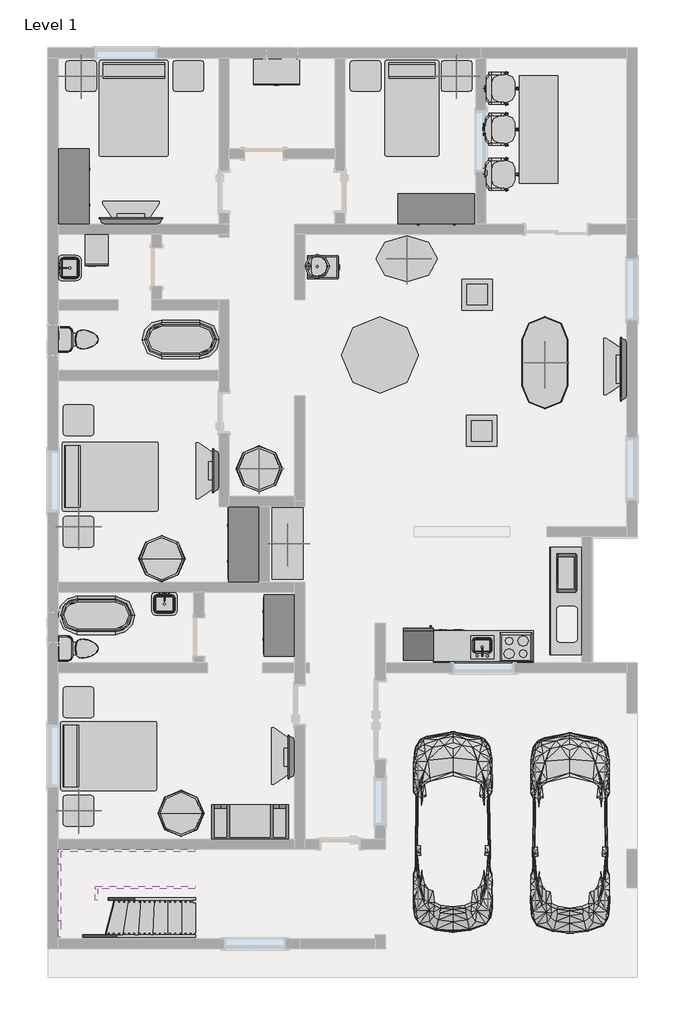
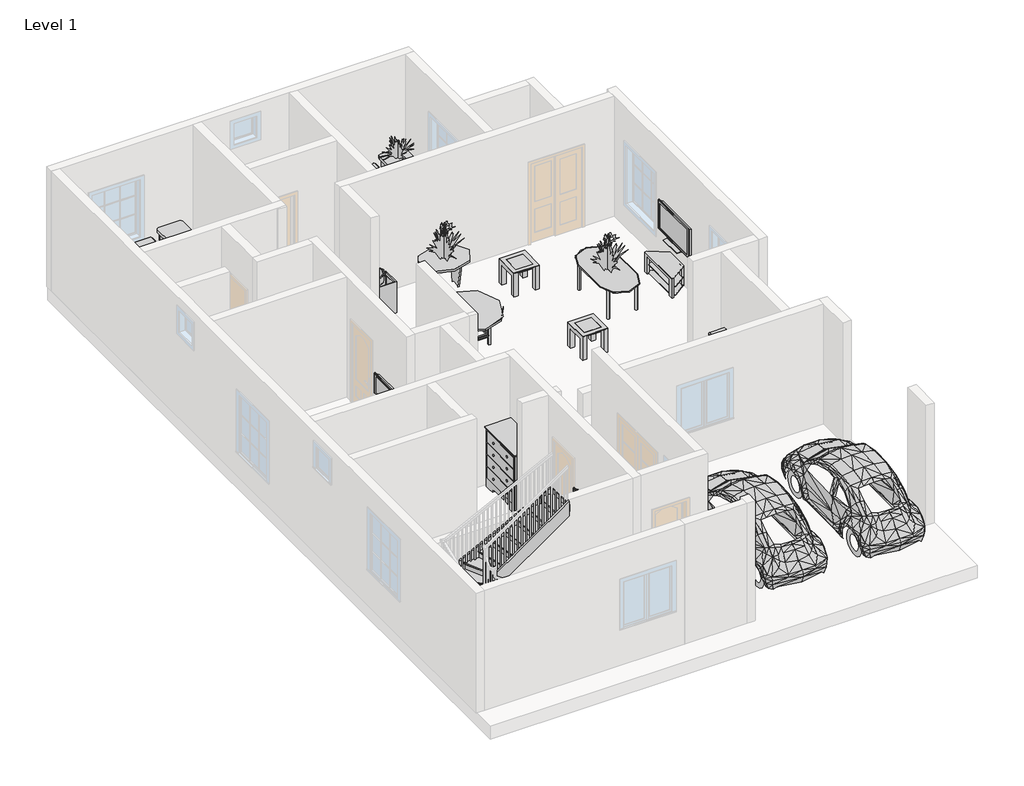
# One storey, part 3 of 3: 42 furniture elements, 8 flow terminals, 8 geographic elements, 8 members, 8 proxies, 1 stair flight.
"""IFC4 building model written with IfcOpenShell, lengths in millimetres."""

from ifc_helpers import new_model, si_unit, frame, origin, place, context, project, spatial, polyline, outline, extrude, transform, mapped, element, save
from components import proxy_7e1014cc, proxy_a6faaae8, proxy_45b28599, kitchenette_medium_kitchenette_medium_844211aa, proxy_8a8d5ab2, rpc_beetle_rpc_beetle_3ce7ba48, proxy_c523a7b7, flow_terminal_871c2e40, flow_terminal_d49f872f, flow_terminal_62a433f7, toilet_domestic_3d_toilet_domestic_3d_f7549cf7, toilet_domestic_3d_toilet_domestic_3d_183bbd19, flow_terminal_b374fae2, furniture_3e5ce493, furniture_0253826f, furniture_c3d8c53b, chair_executive_chair_executive_8d69e98c, furniture_c6510c7c, furniture_ac03d711, furniture_2babcf72, furniture_d0678273, furniture_cdca18a6, furniture_e1dba61b, furniture_56245f3a, furniture_fdf74506, tv_stand_tv_stand_6ce107e5, furniture_b5c51a22, furniture_92191dda, furniture_2c34a4f9, furniture_bbcc68ce, furniture_cd2394ed, furniture_bcf351fa, furniture_0d1ceb4d, furniture_c80d6d9c, rpc_plant_tropical_55f6ff97, rpc_plant_tropical_agave_1_5_93a2a214, rpc_plant_tropical_dagger_2_80c14bd7, stair_flight_7ceb0e75

model = new_model("IFC4")

# Units and contexts
model_context = context("Model", 3, world=origin())
ifc_project = project(units=[si_unit("LENGTHUNIT", "METRE", prefix="MILLI")], contexts=[model_context])

# Site, building, storey
site = spatial("IfcSite", under=ifc_project)
building = spatial("IfcBuilding", under=site)
storey = spatial("IfcBuildingStorey", under=building, Name="Level 1", Elevation=0.0)

# Proxies
placement = place(None, origin())
proxy_shape = proxy_7e1014cc(model_context)
element("IfcBuildingElementProxy", 1, Name="18\" x 24\" x 34 1/2\"", ObjectType="18\" x 24\" x 34 1/2\"", at=placement, inside=storey, context=model_context, shape_type="MappedRepresentation", body=[
    mapped(proxy_shape, transform((-12910.2486815, 9726.4137408, 0.0), x_axis=(1.0, 0.0, 0.0), y_axis=(0.0, 1.0, 0.0), z_axis=(0.0, 0.0, 1.0))),
])
proxy_2_shape = proxy_a6faaae8(model_context)
element("IfcBuildingElementProxy", 2, Name="Cook Top-4 Unit2 : 22\" x 20\"", ObjectType="Cook Top-4 Unit2 : 22\" x 20\"", at=placement, inside=storey, context=model_context, shape_type="MappedRepresentation", body=[
    mapped(proxy_2_shape, transform((-4274.431213, 2105.6633056, 0.0), x_axis=(-0.9999999999999998, 0.0, 0.0), y_axis=(0.0, -0.9999999999999998, 0.0), z_axis=(0.0, 0.0, 1.0))),
])
proxy_3_shape = proxy_45b28599(model_context)
element("IfcBuildingElementProxy", 3, Name="Dishwasher : 24\" x 24\" x 34\"", ObjectType="Dishwasher : 24\" x 24\" x 34\"", at=placement, inside=storey, context=model_context, shape_type="MappedRepresentation", body=[
    mapped(proxy_3_shape, transform((-5225.6137445, 2397.5128704, 0.0), x_axis=(-0.9999999999999998, 0.0, 0.0), y_axis=(0.0, -0.9999999999999998, 0.0), z_axis=(0.0, 0.0, 1.0))),
])
kitchenette_medium_kitchenette_medium_shape = kitchenette_medium_kitchenette_medium_844211aa(model_context)
element("IfcBuildingElementProxy", 4, Name="Kitchenette - Medium : Kitchenette - Medium", ObjectType="Kitchenette - Medium : Kitchenette - Medium", at=placement, inside=storey, context=model_context, shape_type="MappedRepresentation", body=[
    mapped(kitchenette_medium_kitchenette_medium_shape, transform((-4598.5935081, 1800.8633056, 0.0), x_axis=(-0.9999999999999998, 0.0, 0.0), y_axis=(0.0, -0.9999999999999998, 0.0), z_axis=(0.0, 0.0, 1.0))),
])
proxy_4_shape = proxy_8a8d5ab2(model_context)
element("IfcBuildingElementProxy", 5, Name="Microwave : 30\" x 16\" x 18\"", ObjectType="Microwave : 30\" x 16\" x 18\"", at=placement, inside=storey, context=model_context, shape_type="MappedRepresentation", body=[
    mapped(proxy_4_shape, transform((-2912.7507072, 4078.956183, 0.0), x_axis=(0.0, -1.0000000000000004, 0.0), y_axis=(1.0000000000000004, 0.0, 0.0), z_axis=(0.0, 0.0, 1.0))),
])
rpc_beetle_rpc_beetle_shape = rpc_beetle_rpc_beetle_3ce7ba48(model_context)
element("IfcBuildingElementProxy", 6, Name="RPC Beetle : RPC Beetle", ObjectType="RPC Beetle : RPC Beetle", at=placement, inside=storey, context=model_context, shape_type="MappedRepresentation", body=[
    mapped(rpc_beetle_rpc_beetle_shape, transform((-5530.931213, -2791.3366944, 0.0), x_axis=(1.0, 0.0, 0.0), y_axis=(0.0, 1.0, 0.0), z_axis=(0.0, 0.0, 1.0))),
])
element("IfcBuildingElementProxy", 7, Name="RPC Beetle : RPC Beetle", ObjectType="RPC Beetle : RPC Beetle", at=placement, inside=storey, context=model_context, shape_type="MappedRepresentation", body=[
    mapped(rpc_beetle_rpc_beetle_shape, transform((-3202.331213, -2816.7366944, 0.0), x_axis=(1.0, 0.0, 0.0), y_axis=(0.0, 1.0, 0.0), z_axis=(0.0, 0.0, 1.0))),
])
proxy_5_shape = proxy_c523a7b7(model_context)
element("IfcBuildingElementProxy", 8, Name="Refrigerator : 24\" x 25\" LH", ObjectType="Refrigerator : 24\" x 25\" LH", at=placement, inside=storey, context=model_context, shape_type="MappedRepresentation", body=[
    mapped(proxy_5_shape, transform((-6211.181213, 2151.3122771, 0.0), x_axis=(-0.9999999999999998, 0.0, 0.0), y_axis=(0.0, -0.9999999999999998, 0.0), z_axis=(0.0, 0.0, 1.0))),
])

# Flow terminals
flow_terminal_shape = flow_terminal_871c2e40(model_context)
element("IfcFlowTerminal", 9, ObjectType="Sink Kitchen-Island : 18\" x 18\"", at=placement, inside=storey, context=model_context, shape_type="MappedRepresentation", body=[
    mapped(flow_terminal_shape, transform((-4931.8419724, 2108.0087067, -14.4), x_axis=(-0.9999999999999998, 0.0, 0.0), y_axis=(0.0, -0.9999999999999998, 0.0), z_axis=(0.0, 0.0, 1.0))),
])
flow_terminal_2_shape = flow_terminal_d49f872f(model_context)
element("IfcFlowTerminal", 10, ObjectType="Sink Vanity-Round : 19\" x 19\"", at=placement, inside=storey, context=model_context, shape_type="MappedRepresentation", body=[
    mapped(flow_terminal_2_shape, transform((-8139.9877856, 9566.0115651, 304.8), x_axis=(0.0, 1.0000000000000002, 0.0), y_axis=(-1.0000000000000002, 0.0, 0.0), z_axis=(0.0, 0.0, 1.0))),
])
flow_terminal_3_shape = flow_terminal_62a433f7(model_context)
element("IfcFlowTerminal", 11, ObjectType="Sink Vanity-Square : 20\" x 18\"", at=placement, inside=storey, context=model_context, shape_type="MappedRepresentation", body=[
    mapped(flow_terminal_3_shape, transform((-13190.3858119, 9616.3740651, 0.0), x_axis=(0.0, 1.0000000000000002, 0.0), y_axis=(-1.0000000000000002, 0.0, 0.0), z_axis=(0.0, 0.0, 1.0))),
])
element("IfcFlowTerminal", 12, ObjectType="Sink Vanity-Square : 20\" x 18\"", at=placement, inside=storey, context=model_context, shape_type="MappedRepresentation", body=[
    mapped(flow_terminal_3_shape, transform((-11273.6204535, 3017.5179045, 0.0), x_axis=(1.0000000000000002, 0.0, 0.0), y_axis=(0.0, 1.0000000000000002, 0.0), z_axis=(0.0, 0.0, 1.0))),
])
toilet_domestic_3d_toilet_domestic_3d_shape = toilet_domestic_3d_toilet_domestic_3d_f7549cf7(model_context)
toilet_domestic_3d_toilet_domestic_3d_2_shape = toilet_domestic_3d_toilet_domestic_3d_183bbd19(model_context)
element("IfcFlowTerminal", 13, ObjectType="Toilet-Domestic-3D : Toilet-Domestic-3D", at=placement, inside=storey, context=model_context, shape_type="MappedRepresentation", body=[
    mapped(toilet_domestic_3d_toilet_domestic_3d_shape, transform((-12875.8351856, 2080.0633056, 0.0), x_axis=(0.0, 1.0000000000000002, 0.0), y_axis=(-1.0000000000000002, 0.0, 0.0), z_axis=(0.0, 0.0, 1.0))),
    mapped(toilet_domestic_3d_toilet_domestic_3d_2_shape, transform((-12875.8351856, 2080.0633056, 0.0), x_axis=(0.0, 1.0000000000000002, 0.0), y_axis=(-1.0000000000000002, 0.0, 0.0), z_axis=(0.0, 0.0, 1.0))),
])
element("IfcFlowTerminal", 14, ObjectType="Toilet-Domestic-3D : Toilet-Domestic-3D", at=placement, inside=storey, context=model_context, shape_type="MappedRepresentation", body=[
    mapped(toilet_domestic_3d_toilet_domestic_3d_shape, transform((-12875.8351856, 8213.4633056, 0.0), x_axis=(0.0, 1.0000000000000002, 0.0), y_axis=(-1.0000000000000002, 0.0, 0.0), z_axis=(0.0, 0.0, 1.0))),
    mapped(toilet_domestic_3d_toilet_domestic_3d_2_shape, transform((-12875.8351856, 8213.4633056, 0.0), x_axis=(0.0, 1.0000000000000002, 0.0), y_axis=(-1.0000000000000002, 0.0, 0.0), z_axis=(0.0, 0.0, 1.0))),
])
flow_terminal_4_shape = flow_terminal_b374fae2(model_context)
element("IfcFlowTerminal", 15, ObjectType="Tub-Free Standing-3D : 30\" x 60\"", at=placement, inside=storey, context=model_context, shape_type="MappedRepresentation", body=[
    mapped(flow_terminal_4_shape, transform((-12608.531213, 2740.4633056, 0.0), x_axis=(0.0, 1.0000000000000002, 0.0), y_axis=(-1.0000000000000002, 0.0, 0.0), z_axis=(0.0, 0.0, 1.0))),
])
element("IfcFlowTerminal", 16, ObjectType="Tub-Free Standing-3D : 30\" x 60\"", at=placement, inside=storey, context=model_context, shape_type="MappedRepresentation", body=[
    mapped(flow_terminal_4_shape, transform((-10935.731213, 8213.4633056, 0.0), x_axis=(0.0, -1.0000000000000004, 0.0), y_axis=(1.0000000000000004, 0.0, 0.0), z_axis=(0.0, 0.0, 1.0))),
])

# Furniture
furniture_shape = furniture_3e5ce493(model_context)
element("IfcFurniture", 17, ObjectType="Base Cabinet-2 Bin : 18\"", at=placement, inside=storey, context=model_context, shape_type="MappedRepresentation", body=[
    mapped(furniture_shape, transform((-8419.731213, 9631.2256007, 0.0), x_axis=(0.0, 1.0, 0.0), y_axis=(-1.0, 0.0, 0.0), z_axis=(0.0, 0.0, 1.0))),
])
furniture_2_shape = furniture_0253826f(model_context)
element("IfcFurniture", 18, ObjectType="Bed-Standard.0001 : Double 54\" x 75\"", at=placement, inside=storey, context=model_context, shape_type="MappedRepresentation", body=[
    mapped(furniture_2_shape, transform((-12139.0197376, 12846.5583876, 0.0), x_axis=(1.0, 0.0, 0.0), y_axis=(0.0, 1.0, 0.0), z_axis=(0.0, 0.0, 1.0))),
])
element("IfcFurniture", 19, ObjectType="Bed-Standard.0001 : Double 54\" x 75\"", at=placement, inside=storey, context=model_context, shape_type="MappedRepresentation", body=[
    mapped(furniture_2_shape, transform((-12383.0262949, 5219.974781, 0.0), x_axis=(0.0, 1.0, 0.0), y_axis=(-1.0, 0.0, 0.0), z_axis=(0.0, 0.0, 1.0))),
])
element("IfcFurniture", 20, ObjectType="Bed-Standard.0001 : Double 54\" x 75\"", at=placement, inside=storey, context=model_context, shape_type="MappedRepresentation", body=[
    mapped(furniture_2_shape, transform((-12412.8262949, -324.825219, 0.0), x_axis=(0.0, 1.0000000000000002, 0.0), y_axis=(-1.0000000000000002, 0.0, 0.0), z_axis=(0.0, 0.0, 1.0))),
])
furniture_3_shape = furniture_c3d8c53b(model_context)
element("IfcFurniture", 21, ObjectType="Bed-Standard.0001 : Twin 38\" x 75\"", at=placement, inside=storey, context=model_context, shape_type="MappedRepresentation", body=[
    mapped(furniture_3_shape, transform((-6615.2197376, 12846.5583876, 0.0), x_axis=(1.0, 0.0, 0.0), y_axis=(0.0, 1.0, 0.0), z_axis=(0.0, 0.0, 1.0))),
])
chair_executive_chair_executive_shape = chair_executive_chair_executive_8d69e98c(model_context)
element("IfcFurniture", 22, ObjectType="Chair-Executive : Chair-Executive", at=placement, inside=storey, context=model_context, shape_type="MappedRepresentation", body=[
    mapped(chair_executive_chair_executive_shape, transform((-4581.8771146, 11632.4541253, 0.0), x_axis=(0.0, -1.0000000000000004, 0.0), y_axis=(1.0000000000000004, 0.0, 0.0), z_axis=(0.0, 0.0, 1.0))),
])
element("IfcFurniture", 23, ObjectType="Chair-Executive : Chair-Executive", at=placement, inside=storey, context=model_context, shape_type="MappedRepresentation", body=[
    mapped(chair_executive_chair_executive_shape, transform((-4581.8771146, 12522.8541253, 0.0), x_axis=(0.0, -1.0, 0.0), y_axis=(1.0, 0.0, 0.0), z_axis=(0.0, 0.0, 1.0))),
])
element("IfcFurniture", 24, ObjectType="Chair-Executive : Chair-Executive", at=placement, inside=storey, context=model_context, shape_type="MappedRepresentation", body=[
    mapped(chair_executive_chair_executive_shape, transform((-4581.8771146, 13335.6541253, 0.0), x_axis=(0.0, -1.0, 0.0), y_axis=(1.0, 0.0, 0.0), z_axis=(0.0, 0.0, 1.0))),
])
furniture_4_shape = furniture_c6510c7c(model_context)
element("IfcFurniture", 25, ObjectType="Counter Top w Sink Hole : 24\" Depth", at=placement, inside=storey, context=model_context, shape_type="MappedRepresentation", body=[
    mapped(furniture_4_shape, transform((-5131.9935081, 1800.8633056, -14.4), x_axis=(-0.9999999999999998, 0.0, 0.0), y_axis=(0.0, -0.9999999999999998, 0.0), z_axis=(0.0, 0.0, 1.0))),
])
furniture_5_shape = furniture_ac03d711(model_context)
element("IfcFurniture", 26, ObjectType="Counter Top w Sink Hole : 24\" Depth", at=placement, inside=storey, context=model_context, shape_type="MappedRepresentation", body=[
    mapped(furniture_5_shape, transform((-3608.731213, 3153.7256007, 0.0), x_axis=(0.0, 1.0, 0.0), y_axis=(-1.0, 0.0, 0.0), z_axis=(0.0, 0.0, 1.0))),
])
furniture_6_shape = furniture_2babcf72(model_context)
element("IfcFurniture", 27, ObjectType="Dresser : 48\" x 60\" x 24\"", at=placement, inside=storey, context=model_context, shape_type="MappedRepresentation", body=[
    mapped(furniture_6_shape, transform((-8615.3682589, 2268.0700458, 0.0), x_axis=(0.0, -1.0000000000000007, 0.0), y_axis=(1.0000000000000007, 0.0, 0.0), z_axis=(0.0, 0.0, 1.0))),
])
furniture_7_shape = furniture_d0678273(model_context)
element("IfcFurniture", 28, ObjectType="Dresser : 48\" x 72\" x 24\"", at=placement, inside=storey, context=model_context, shape_type="MappedRepresentation", body=[
    mapped(furniture_7_shape, transform((-13424.4941671, 11506.6565655, 0.0), x_axis=(0.0, 1.000000000000001, 0.0), y_axis=(-1.000000000000001, 0.0, 0.0), z_axis=(0.0, 0.0, 1.0))),
])
element("IfcFurniture", 29, ObjectType="Dresser : 48\" x 72\" x 24\"", at=placement, inside=storey, context=model_context, shape_type="MappedRepresentation", body=[
    mapped(furniture_7_shape, transform((-5591.9379531, 11168.8262597, 0.0), x_axis=(1.0000000000000009, 0.0, 0.0), y_axis=(0.0, 1.0000000000000009, 0.0), z_axis=(0.0, 0.0, 1.0))),
])
element("IfcFurniture", 30, ObjectType="Dresser : 48\" x 72\" x 24\"", at=placement, inside=storey, context=model_context, shape_type="MappedRepresentation", body=[
    mapped(furniture_7_shape, transform((-9315.3682589, 3893.6700458, 0.0), x_axis=(0.0, -1.0000000000000007, 0.0), y_axis=(1.0000000000000007, 0.0, 0.0), z_axis=(0.0, 0.0, 1.0))),
])
furniture_8_shape = furniture_cdca18a6(model_context)
element("IfcFurniture", 31, ObjectType="Entertainment Center : 72\" x 72\" x 24\"", at=placement, inside=storey, context=model_context, shape_type="MappedRepresentation", body=[
    mapped(furniture_8_shape, transform((-9556.131213, -1800.7366944, 0.0), x_axis=(-1.0000000000000004, 0.0, 0.0), y_axis=(0.0, -1.0000000000000004, 0.0), z_axis=(0.0, 0.0, 1.0))),
])
furniture_9_shape = furniture_e1dba61b(model_context)
element("IfcFurniture", 32, ObjectType="Storage Pedestal : 20\" x 36\" x 36\"", at=placement, inside=storey, context=model_context, shape_type="MappedRepresentation", body=[
    mapped(furniture_9_shape, transform((-8849.308699, 14452.5816817, 0.0), x_axis=(1.0, 0.0, 0.0), y_axis=(0.0, 1.0, 0.0), z_axis=(0.0, 0.0, 1.0))),
])
furniture_10_shape = furniture_56245f3a(model_context)
element("IfcFurniture", 33, ObjectType="TV - Flat Screen : 32\"", at=placement, inside=storey, context=model_context, shape_type="MappedRepresentation", body=[
    mapped(furniture_10_shape, transform((-8732.2698366, -77.4812085, 914.4), x_axis=(0.0, -1.0000000000000004, 0.0), y_axis=(1.0000000000000004, 0.0, 0.0), z_axis=(0.0, 0.0, 1.0))),
])
element("IfcFurniture", 34, ObjectType="TV - Flat Screen : 32\"", at=placement, inside=storey, context=model_context, shape_type="MappedRepresentation", body=[
    mapped(furniture_10_shape, transform((-10232.2698366, 5604.9187915, 914.4), x_axis=(0.0, -1.0000000000000004, 0.0), y_axis=(1.0000000000000004, 0.0, 0.0), z_axis=(0.0, 0.0, 1.0))),
])
furniture_11_shape = furniture_fdf74506(model_context)
element("IfcFurniture", 35, ObjectType="TV - Flat Screen : 50\"", at=placement, inside=storey, context=model_context, shape_type="MappedRepresentation", body=[
    mapped(furniture_11_shape, transform((-11926.6757271, 10559.4019293, 914.4), x_axis=(-1.0000000000000004, 0.0, 0.0), y_axis=(0.0, -1.0000000000000004, 0.0), z_axis=(0.0, 0.0, 1.0))),
])
element("IfcFurniture", 36, ObjectType="TV - Flat Screen : 50\"", at=placement, inside=storey, context=model_context, shape_type="MappedRepresentation", body=[
    mapped(furniture_11_shape, transform((-2132.2698366, 7621.1187915, 914.4), x_axis=(0.0, -1.0000000000000004, 0.0), y_axis=(1.0000000000000004, 0.0, 0.0), z_axis=(0.0, 0.0, 1.0))),
])
tv_stand_tv_stand_shape = tv_stand_tv_stand_6ce107e5(model_context)
element("IfcFurniture", 37, ObjectType="TV Stand : TV Stand", at=placement, inside=storey, context=model_context, shape_type="MappedRepresentation", body=[
    mapped(tv_stand_tv_stand_shape, transform((-8673.731213, 71.8513077, 0.0), x_axis=(0.0, -1.0000000000000002, 0.0), y_axis=(1.0000000000000002, 0.0, 0.0), z_axis=(0.0, 0.0, 1.0))),
])
element("IfcFurniture", 38, ObjectType="TV Stand : TV Stand", at=placement, inside=storey, context=model_context, shape_type="MappedRepresentation", body=[
    mapped(tv_stand_tv_stand_shape, transform((-11797.5432109, 10500.8633056, 0.0), x_axis=(-1.0000000000000002, 0.0, 0.0), y_axis=(0.0, -1.0000000000000002, 0.0), z_axis=(0.0, 0.0, 1.0))),
])
element("IfcFurniture", 39, ObjectType="TV Stand : TV Stand", at=placement, inside=storey, context=model_context, shape_type="MappedRepresentation", body=[
    mapped(tv_stand_tv_stand_shape, transform((-10173.731213, 5734.0513077, 0.0), x_axis=(0.0, -1.0000000000000004, 0.0), y_axis=(1.0000000000000004, 0.0, 0.0), z_axis=(0.0, 0.0, 1.0))),
])
element("IfcFurniture", 40, ObjectType="TV Stand : TV Stand", at=placement, inside=storey, context=model_context, shape_type="MappedRepresentation", body=[
    mapped(tv_stand_tv_stand_shape, transform((-2073.731213, 7802.2513077, 0.0), x_axis=(0.0, -0.9999999999999998, 0.0), y_axis=(0.9999999999999998, 0.0, 0.0), z_axis=(0.0, 0.0, 1.0))),
])
furniture_12_shape = furniture_b5c51a22(model_context)
element("IfcFurniture", 41, ObjectType="Table-Coffee : 24\" x 24\" x 24\"", at=placement, inside=storey, context=model_context, shape_type="MappedRepresentation", body=[
    mapped(furniture_12_shape, transform((-4976.9896084, 6307.4022278, 0.0), x_axis=(1.0, 0.0, 0.0), y_axis=(0.0, 1.0, 0.0), z_axis=(0.0, 0.0, 1.0))),
])
element("IfcFurniture", 42, ObjectType="Table-Coffee : 24\" x 24\" x 24\"", at=placement, inside=storey, context=model_context, shape_type="MappedRepresentation", body=[
    mapped(furniture_12_shape, transform((-5063.7969796, 9007.2522278, 0.0), x_axis=(1.0, 0.0, 0.0), y_axis=(0.0, 1.0, 0.0), z_axis=(0.0, 0.0, 1.0))),
])
furniture_13_shape = furniture_92191dda(model_context)
element("IfcFurniture", 43, ObjectType="Table-Dining : 30\" x 84\" x 22\"", at=placement, inside=storey, context=model_context, shape_type="MappedRepresentation", body=[
    mapped(furniture_13_shape, transform((-3733.9201352, 12363.597539, 0.0), x_axis=(0.0, 1.0, 0.0), y_axis=(-1.0, 0.0, 0.0), z_axis=(0.0, 0.0, 1.0))),
])
furniture_14_shape = furniture_2c34a4f9(model_context)
element("IfcFurniture", 44, ObjectType="Table-Dining Oval : 36\" x 72\"", at=placement, inside=storey, context=model_context, shape_type="MappedRepresentation", body=[
    mapped(furniture_14_shape, transform((-4060.2295736, 8155.0829778, 0.0), x_axis=(0.0, 1.0, 0.0), y_axis=(-1.0, 0.0, 0.0), z_axis=(0.0, 0.0, 1.0))),
])
furniture_15_shape = furniture_bbcc68ce(model_context)
element("IfcFurniture", 45, ObjectType="Table-Dining Round w Chairs : 60\" Diameter", at=placement, inside=storey, context=model_context, shape_type="MappedRepresentation", body=[
    mapped(furniture_15_shape, transform((-7082.4131802, 8090.5419941, 0.0), x_axis=(1.0, 0.0, 0.0), y_axis=(0.0, 1.0, 0.0), z_axis=(0.0, 0.0, 1.0))),
])
furniture_16_shape = furniture_cd2394ed(model_context)
element("IfcFurniture", 46, ObjectType="Table-Ellipse : 72\" x 36\"", at=placement, inside=storey, context=model_context, shape_type="MappedRepresentation", body=[
    mapped(furniture_16_shape, transform((-6445.331213, 9815.0633056, 0.0), x_axis=(1.0, 0.0, 0.0), y_axis=(0.0, 1.0, 0.0), z_axis=(0.0, 0.0, 1.0))),
])
furniture_17_shape = furniture_bcf351fa(model_context)
element("IfcFurniture", 47, ObjectType="Table-End : 24\" x 24\"", at=placement, inside=storey, context=model_context, shape_type="MappedRepresentation", body=[
    mapped(furniture_17_shape, transform((-13272.6648433, 861.0633056, 0.0), x_axis=(1.0, 0.0, 0.0), y_axis=(0.0, 1.0, 0.0), z_axis=(0.0, 0.0, 1.0))),
])
element("IfcFurniture", 48, ObjectType="Table-End : 24\" x 24\"", at=placement, inside=storey, context=model_context, shape_type="MappedRepresentation", body=[
    mapped(furniture_17_shape, transform((-13272.6648433, -1289.9366944, 0.0), x_axis=(1.0, 0.0, 0.0), y_axis=(0.0, 1.0, 0.0), z_axis=(0.0, 0.0, 1.0))),
])
element("IfcFurniture", 49, ObjectType="Table-End : 24\" x 24\"", at=placement, inside=storey, context=model_context, shape_type="MappedRepresentation", body=[
    mapped(furniture_17_shape, transform((-13272.6648433, 4246.8633056, 0.0), x_axis=(1.0, 0.0, 0.0), y_axis=(0.0, 1.0, 0.0), z_axis=(0.0, 0.0, 1.0))),
])
element("IfcFurniture", 50, ObjectType="Table-End : 24\" x 24\"", at=placement, inside=storey, context=model_context, shape_type="MappedRepresentation", body=[
    mapped(furniture_17_shape, transform((-13272.6648433, 6457.8633056, 0.0), x_axis=(1.0, 0.0, 0.0), y_axis=(0.0, 1.0, 0.0), z_axis=(0.0, 0.0, 1.0))),
])
element("IfcFurniture", 51, ObjectType="Table-End : 24\" x 24\"", at=placement, inside=storey, context=model_context, shape_type="MappedRepresentation", body=[
    mapped(furniture_17_shape, transform((-13217.4648433, 13289.6633056, 0.0), x_axis=(1.0, 0.0, 0.0), y_axis=(0.0, 1.0, 0.0), z_axis=(0.0, 0.0, 1.0))),
])
element("IfcFurniture", 52, ObjectType="Table-End : 24\" x 24\"", at=placement, inside=storey, context=model_context, shape_type="MappedRepresentation", body=[
    mapped(furniture_17_shape, transform((-11091.8648433, 13289.6633056, 0.0), x_axis=(1.0, 0.0, 0.0), y_axis=(0.0, 1.0, 0.0), z_axis=(0.0, 0.0, 1.0))),
])
element("IfcFurniture", 53, ObjectType="Table-End : 24\" x 24\"", at=placement, inside=storey, context=model_context, shape_type="MappedRepresentation", body=[
    mapped(furniture_17_shape, transform((-5763.2648433, 13289.6633056, 0.0), x_axis=(1.0, 0.0, 0.0), y_axis=(0.0, 1.0, 0.0), z_axis=(0.0, 0.0, 1.0))),
])
element("IfcFurniture", 54, ObjectType="Table-End : 24\" x 24\"", at=placement, inside=storey, context=model_context, shape_type="MappedRepresentation", body=[
    mapped(furniture_17_shape, transform((-7572.6648433, 13289.6633056, 0.0), x_axis=(1.0, 0.0, 0.0), y_axis=(0.0, 1.0, 0.0), z_axis=(0.0, 0.0, 1.0))),
])
furniture_18_shape = furniture_0d1ceb4d(model_context)
element("IfcFurniture", 55, ObjectType="Table-Rectangular : 72\" x 30\"", at=placement, inside=storey, context=model_context, shape_type="MappedRepresentation", body=[
    mapped(furniture_18_shape, transform((-8814.931213, 4162.8633056, 0.0), x_axis=(0.0, 1.0000000000000002, 0.0), y_axis=(-1.0000000000000002, 0.0, 0.0), z_axis=(0.0, 0.0, 1.0))),
])
furniture_19_shape = furniture_c80d6d9c(model_context)
element("IfcFurniture", 56, ObjectType="Table-Round : 36\" Diameter", at=placement, inside=storey, context=model_context, shape_type="MappedRepresentation", body=[
    mapped(furniture_19_shape, transform((-11308.731213, 3865.8633056, 0.0), x_axis=(1.0, 0.0, 0.0), y_axis=(0.0, 1.0, 0.0), z_axis=(0.0, 0.0, 1.0))),
])
element("IfcFurniture", 57, ObjectType="Table-Round : 36\" Diameter", at=placement, inside=storey, context=model_context, shape_type="MappedRepresentation", body=[
    mapped(furniture_19_shape, transform((-10927.731213, -1188.3366944, 0.0), x_axis=(1.0, 0.0, 0.0), y_axis=(0.0, 1.0, 0.0), z_axis=(0.0, 0.0, 1.0))),
])
element("IfcFurniture", 58, ObjectType="Table-Round : 36\" Diameter", at=placement, inside=storey, context=model_context, shape_type="MappedRepresentation", body=[
    mapped(furniture_19_shape, transform((-9373.731213, 5645.0633056, 0.0), x_axis=(1.0, 0.0, 0.0), y_axis=(0.0, 1.0, 0.0), z_axis=(0.0, 0.0, 1.0))),
])

# Geographic elements
rpc_plant_tropical_shape = rpc_plant_tropical_55f6ff97(model_context)
element("IfcGeographicElement", 59, ObjectType="RPC Plant - Tropical", at=placement, inside=storey, context=model_context, shape_type="MappedRepresentation", body=[
    mapped(rpc_plant_tropical_shape, transform((-3702.131213, 7753.2633056, 762.0), x_axis=(1.0, 0.0, 0.0), y_axis=(0.0, 1.0, 0.0), z_axis=(0.0, 0.0, 1.0))),
])
element("IfcGeographicElement", 60, ObjectType="RPC Plant - Tropical", at=placement, inside=storey, context=model_context, shape_type="MappedRepresentation", body=[
    mapped(rpc_plant_tropical_shape, transform((-9373.731213, 5645.0633056, 762.0), x_axis=(1.0, 0.0, 0.0), y_axis=(0.0, 1.0, 0.0), z_axis=(0.0, 0.0, 1.0))),
])
element("IfcGeographicElement", 61, ObjectType="RPC Plant - Tropical", at=placement, inside=storey, context=model_context, shape_type="MappedRepresentation", body=[
    mapped(rpc_plant_tropical_shape, transform((-6445.331213, 9815.0633056, 762.0), x_axis=(1.0, 0.0, 0.0), y_axis=(0.0, 1.0, 0.0), z_axis=(0.0, 0.0, 1.0))),
])
rpc_plant_tropical_agave_1_5_shape = rpc_plant_tropical_agave_1_5_93a2a214(model_context)
element("IfcGeographicElement", 62, ObjectType="RPC Plant - Tropical : Agave - 1.5'", at=placement, inside=storey, context=model_context, shape_type="MappedRepresentation", body=[
    mapped(rpc_plant_tropical_agave_1_5_shape, transform((-12964.131213, -1137.5366944, 762.0), x_axis=(1.0, 0.0, 0.0), y_axis=(0.0, 1.0, 0.0), z_axis=(0.0, 0.0, 1.0))),
])
element("IfcGeographicElement", 63, ObjectType="RPC Plant - Tropical : Agave - 1.5'", at=placement, inside=storey, context=model_context, shape_type="MappedRepresentation", body=[
    mapped(rpc_plant_tropical_agave_1_5_shape, transform((-12964.131213, 4500.8633056, 762.0), x_axis=(1.0, 0.0, 0.0), y_axis=(0.0, 1.0, 0.0), z_axis=(0.0, 0.0, 1.0))),
])
element("IfcGeographicElement", 64, ObjectType="RPC Plant - Tropical : Agave - 1.5'", at=placement, inside=storey, context=model_context, shape_type="MappedRepresentation", body=[
    mapped(rpc_plant_tropical_agave_1_5_shape, transform((-12908.931213, 13442.0633056, 762.0), x_axis=(1.0, 0.0, 0.0), y_axis=(0.0, 1.0, 0.0), z_axis=(0.0, 0.0, 1.0))),
])
element("IfcGeographicElement", 65, ObjectType="RPC Plant - Tropical : Agave - 1.5'", at=placement, inside=storey, context=model_context, shape_type="MappedRepresentation", body=[
    mapped(rpc_plant_tropical_agave_1_5_shape, transform((-5454.731213, 13442.0633056, 762.0), x_axis=(1.0, 0.0, 0.0), y_axis=(0.0, 1.0, 0.0), z_axis=(0.0, 0.0, 1.0))),
])
rpc_plant_tropical_dagger_2_shape = rpc_plant_tropical_dagger_2_80c14bd7(model_context)
element("IfcGeographicElement", 66, ObjectType="RPC Plant - Tropical : Dagger - 2'", at=placement, inside=storey, context=model_context, shape_type="MappedRepresentation", body=[
    mapped(rpc_plant_tropical_dagger_2_shape, transform((-8814.931213, 4162.8633056, 762.0), x_axis=(1.0, 0.0, 0.0), y_axis=(0.0, 1.0, 0.0), z_axis=(0.0, 0.0, 1.0))),
])

# Members
element("IfcMember", 67, ObjectType="Stringer - 2\" Width", at=placement, inside=storey, context=model_context, shape_type="SweptSolid", body=[
    extrude(outline(polyline([(58.2684498, -10636.560337), (400.2687254, -10636.560337), (1765.7682263, -13319.731213), (1423.7679507, -13319.731213), (58.2684498, -10636.560337)])), frame((0.0, -3649.9366944, 0.0), z_axis=(0.0, 1.0, 0.0), x_axis=(0.0, 0.0, 1.0)), (0.0, 0.0, 1.0), 50.8),
])
element("IfcMember", 68, ObjectType="Stringer - 2\" Width", at=placement, inside=storey, context=model_context, shape_type="SweptSolid", body=[
    extrude(outline(polyline([(-13319.731213, -3649.9366944), (-13370.531213, -3649.9366944), (-13370.531213, -3323.7635494), (-13319.731213, -3323.7635494), (-13319.731213, -3649.9366944)])), frame((0.0, 0.0, 1423.7679507), z_axis=(0.0, 0.0, 1.0), x_axis=(1.0, 0.0, 0.0)), (0.0, 0.0, 1.0), 342.0002756),
])
element("IfcMember", 69, ObjectType="Stringer - 2\" Width", at=placement, inside=storey, context=model_context, shape_type="SweptSolid", body=[
    extrude(outline(polyline([(-3323.7635494, 1423.7679507), (-3323.7635494, 1765.7682263), (-2202.045892, 2215.1936068), (-2202.045892, 1873.1933311), (-3323.7635494, 1423.7679507)])), frame((-13370.531213, 0.0, 0.0), z_axis=(1.0, 0.0, 0.0), x_axis=(0.0, 1.0, 0.0)), (0.0, 0.0, 1.0), 50.8),
])
element("IfcMember", 70, ObjectType="Stringer - 2\" Width", at=placement, inside=storey, context=model_context, shape_type="SweptSolid", body=[
    extrude(outline(polyline([(-13319.731213, -2202.045892), (-13370.531213, -2202.045892), (-13370.531213, -1948.1366944), (-13319.731213, -1948.1366944), (-13319.731213, -2202.045892)])), frame((0.0, 0.0, 1879.4733394), z_axis=(0.0, 0.0, 1.0), x_axis=(1.0, 0.0, 0.0)), (0.0, 0.0, 1.0), 328.3542079),
])
element("IfcMember", 71, ObjectType="Stringer - 2\" Width", at=placement, inside=storey, context=model_context, shape_type="SweptSolid", body=[
    extrude(outline(polyline([(2182.2271316, -13370.531213), (1903.0275474, -13370.531213), (1903.0275474, -13272.9915907), (3226.2075954, -10647.3488243), (3554.5618033, -10647.3488243), (2182.2271316, -13370.531213)])), frame((0.0, -1948.1366944, 0.0), z_axis=(0.0, 1.0, 0.0), x_axis=(0.0, 0.0, 1.0)), (0.0, 0.0, 1.0), 50.8),
])
element("IfcMember", 72, ObjectType="Stringer - 2\" Width", at=placement, inside=storey, context=model_context, shape_type="SweptSolid", body=[
    extrude(outline(polyline([(0.0, -10636.560337), (365.6929581, -10636.560337), (1716.0741306, -12583.131213), (1345.1121529, -12583.131213), (0.0, -10644.1556149), (0.0, -10636.560337)])), frame((0.0, -2913.3366944, 0.0), z_axis=(0.0, 1.0, 0.0), x_axis=(0.0, 0.0, 1.0)), (0.0, 0.0, 1.0), 50.8),
])
element("IfcMember", 73, ObjectType="Stringer - 2\" Width", at=placement, inside=storey, context=model_context, shape_type="SweptSolid", body=[
    extrude(outline(polyline([(-2913.3366944, 1412.9559572), (-2913.3366944, 1899.3118054), (-2684.7366944, 2183.5597978), (-2684.7366944, 1697.2039497), (-2913.3366944, 1412.9559572)])), frame((-12633.931213, 0.0, 0.0), z_axis=(1.0, 0.0, 0.0), x_axis=(0.0, 1.0, 0.0)), (0.0, 0.0, 1.0), 50.8),
])
element("IfcMember", 74, ObjectType="Stringer - 2\" Width", at=placement, inside=storey, context=model_context, shape_type="SweptSolid", body=[
    extrude(outline(polyline([(2249.6181171, -12633.931213), (1878.193771, -12633.931213), (3261.6120179, -10647.3488243), (3633.0363641, -10647.3488243), (2249.6181171, -12633.931213)])), frame((0.0, -2684.7366944, 0.0), z_axis=(0.0, 1.0, 0.0), x_axis=(0.0, 0.0, 1.0)), (0.0, 0.0, 1.0), 50.8),
])

# Stair flight
stair_flight_shape = stair_flight_7ceb0e75(model_context)
element("IfcStairFlight", 75, ObjectType="2\" Tread 1\" Nosing 1/4\" Riser", at=placement, inside=storey, context=model_context, shape_type="MappedRepresentation", body=[
    mapped(stair_flight_shape, transform((0.0, 0.0, 0.0), x_axis=(1.0, 0.0, 0.0), y_axis=(0.0, 1.0, 0.0), z_axis=(0.0, 0.0, 1.0))),
])

save(model, "model.ifc")

# Revit data of these elements
# Type "18\" x 24\" x 34 1/2\""
#   Label = "T"
#   Assembly Code = "E1090400"
#   Depth = 2' - 0"
#   Height = 2' - 10 1/2"
#   Width = 1' - 6"
#   Panel Face Material = Plastic, Opaque Black
#   Trach Compact. Material = Steel, Paint Finish, Ivory, Matte
#   Default Elevation = 0
# Type "Cook Top-4 Unit2 : 22\" x 20\""
#   Depth = 1' - 8"
#   Width = 1' - 10"
#   Burner Material = Steel, Chrome Plated
#   Cooktop Material = Steel, Polished
#   Default Elevation = 0
#   Assembly Code = ""
# Type "Dishwasher : 24\" x 24\" x 34\""
#   Label = "DW"
#   Assembly Code = "E1090400"
#   Depth = 2' - 0"
#   Height = 2' - 10"
#   Width = 2' - 0"
#   Dishwasher Material = Steel, Paint Finish, Ivory, Glossy
#   Panel Face Material = Plastic, Opaque Black
#   Default Elevation = 0
# Type "Kitchenette - Medium : Kitchenette - Medium"
#   Assembly Code = "E1090400"
#   Counter Length = 6' - 6"
#   Cabinet Width = 4' - 6"
#   Cabinet Height = 2' - 10 1/2"
#   Cabinet Depth = 2' - 0"
#   Toe Depth = 0' - 3"
#   Toe Height = 0' - 3 1/2"
#   Cabinet Material = Cabinets
#   Door/Drawer Material = Cabinets
#   Handle Material = Cabinets - Handles
#   Default Elevation = 0
# Type "Microwave : 30\" x 16\" x 18\""
#   Assembly Code = "E1090400"
#   Depth = 1' - 4"
#   Height = 1' - 6"
#   Width = 2' - 6"
#   Microwave Material = Laminate, Ivory, Matte
#   Default Elevation = 0
# Type "RPC Beetle : RPC Beetle"
#   built-in parameter 1005195 = "RPC-16-0U6E-L4EG-ENH1-J3KF-SVEL-0TX4-C0"
#   Height = 0
# Type "Refrigerator : 24\" x 25\" LH"
#   Label = "REF."
#   Assembly Code = "E1090400"
#   Depth = 2' - 0 3/4"
#   Handle = 0' - 1 1/2"
#   Height = 5' - 3 1/2"
#   Rear Clearance = 0' - 2"
#   Top Door Height = 1' - 8"
#   Width = 1' - 11 1/2"
#   Material = Steel, Paint Finish, Ivory, Glossy
#   Default Elevation = 0
# Type "Sink Kitchen-Island : 18\" x 18\""
#   Assembly Code = "D2010410"
#   Counter Height = 3' - 0"
#   Depth = 1' - 6"
#   Width = 1' - 6"
#   Faucet Material = Steel, Polished
#   Sink Material = Steel, Polished
#   Default Elevation = 0
# Type "Sink Vanity-Round : 19\" x 19\""
#   Assembly Code = "D2010400"
#   Top Of Counter = 2' - 7"
#   Basin Material = Porcelain, Linen
#   Faucet Material = Steel, Polished
#   Default Elevation = 0
# Type "Sink Vanity-Square : 20\" x 18\""
#   Assembly Code = "D2010400"
#   Counter Height = 2' - 7"
#   Depth = 1' - 6"
#   Width = 1' - 8"
#   Basin Material = Porcelain, Linen
#   Faucet Material = Steel, Polished
#   Default Elevation = 0
# Type "Toilet-Domestic-3D : Toilet-Domestic-3D"
#   Assembly Code = "D2010110"
#   Toilet - Bowl/Basin Material = Porcelain, Linen
#   Toilet - Seat Material = Laminate, Linen, Matte
#   Default Elevation = 0
# Type "Tub-Free Standing-3D : 30\" x 60\""
#   Assembly Code = "D2010110"
#   Height = 1' - 6"
#   Length = 5' - 0"
#   Width = 2' - 6"
#   Tub Material = Porcelain, Ivory
#   Default Elevation = 0
# Type "Base Cabinet-2 Bin : 18\""
#   Assembly Code = "C1030410"
#   Depth = 2' - 0"
#   Height = 2' - 10 1/2"
#   Toe Depth = 0' - 3"
#   Toe Height = 0' - 3 1/2"
#   Width = 1' - 6"
#   Cabinet Material = none
#   Door/Drawer Material = none
#   Handle Material = Cabinets - Handles
#   Panels = none
#   Default Elevation = 0
# Type "Bed-Standard.0001 : Double 54\" x 75\""
#   Assembly Code = "E2020200"
#   Length = 6' - 3"
#   Width = 4' - 6"
#   Leg Material = Steel, Chrome Plated
#   Mattress Material = Linen, White
#   Default Elevation = 0
# Type "Bed-Standard.0001 : Twin 38\" x 75\""
#   Assembly Code = "E2020200"
#   Length = 6' - 3"
#   Width = 3' - 6"
#   Leg Material = Steel, Chrome Plated
#   Mattress Material = Linen, White
#   Default Elevation = 0
# Type "Chair-Executive : Chair-Executive"
#   Assembly Code = "E2020200"
#   Base/Arms Material = Plastic, Opaque Black
#   Casters Material = Plastic, Opaque Black
#   Seat/Back Material = Textile - Slate Blue
#   Default Elevation = 0
# Type "Counter Top w Sink Hole : 24\" Depth"
#   Assembly Code = "C1030400"
#   Counter Thickness = 0' - 1 1/2"
#   Depth = 2' - 1"
#   Height = 3' - 0"
#   Length [instance default] = 8' - 0"
#   Sink Location [instance default] = 2' - 0"
#   Sink Location To Wall [instance default] = 0' - 6"
#   Sink Opening Depth [instance default] = 1' - 3"
#   Sink Opening Width [instance default] = 2' - 3"
#   Counter Top Material = none
#   Default Elevation = 0
# Type "Dresser : 48\" x 60\" x 24\""
#   Assembly Code = "E2020200"
#   Depth = 2' - 0"
#   Height = 5' - 0"
#   Width = 4' - 0"
#   Dresser Material = Laminate - Ivory, Glossy
#   Drawer Material = Laminate, Ivory, Matte
#   Knob Material = Cherry
#   Default Elevation = 0
# Type "Dresser : 48\" x 72\" x 24\""
#   Assembly Code = "E2020200"
#   Depth = 2' - 0"
#   Height = 6' - 0"
#   Width = 5' - 0"
#   Dresser Material = Laminate - Ivory, Glossy
#   Drawer Material = Laminate, Ivory, Matte
#   Knob Material = Cherry
#   Default Elevation = 0
# Type "Entertainment Center : 72\" x 72\" x 24\""
#   Assembly Code = "E2020200"
#   Center Width = 2' - 8"
#   Depth = 2' - 0"
#   Height = 6' - 0"
#   Width = 5' - 0"
#   Material = none
#   Default Elevation = 0
# Type "Storage Pedestal : 20\" x 36\" x 36\""
#   Assembly Code = "E2020"
#   Depth = 1' - 8"
#   Height = 3' - 0"
#   Width = 3' - 0"
#   Cabinet Material = Steel, Paint Finish, Ivory, Glossy
#   Handles Material = Steel, Chrome Plated
#   Default Elevation = 0
# Type "TV - Flat Screen : 32\""
#   SinAng = 0' - 0.0193"
#   L = 2' - 3.79372"
#   H = 1' - 3.6354"
#   Thickness = 0' - 4.33071"
#   Diagonal = 2' - 7.88976"
#   CosAng = 0' - 0.03431"
#   Stand [instance default] = yes
#   Default Elevation = 0
# Type "TV - Flat Screen : 50\""
#   SinAng = 0' - 0.0193"
#   L = 3' - 7.57782"
#   H = 2' - 0.51477"
#   Thickness = 0' - 4.33071"
#   Diagonal = 4' - 2"
#   CosAng = 0' - 0.03431"
#   Stand [instance default] = yes
#   Default Elevation = 0
# Type "TV Stand : TV Stand"
#   Depth = 1' - 6"
#   Width = 3' - 8"
#   Height = 1' - 7 1/2"
#   Finish = Melamine - Gray
#   Default Elevation = 0
# Type "Table-Coffee : 24\" x 24\" x 24\""
#   Assembly Code = "E2020200"
#   Height = 2' - 0"
#   Length = 2' - 0"
#   Width = 2' - 0"
#   Top Material = none
#   Frame Material = none
#   Default Elevation = 0
# Type "Table-Dining : 30\" x 84\" x 22\""
#   Assembly Code = "E2020200"
#   Height = 1' - 10"
#   Length = 7' - 0"
#   Width = 2' - 6"
#   Base Material = Steel, Chrome Plated
#   Top Material = Glass - Clear, Grey
#   Default Elevation = 0
# Type "Table-Dining Oval : 36\" x 72\""
#   Assembly Code = "E2020200"
#   Length = 6' - 0"
#   Width = 3' - 0"
#   Base Material = Steel, Chrome Plated
#   Top Material = Glass - Clear, Grey
#   Default Elevation = 0
#   Description = (empty or 0)
# Type "Table-Dining Round w Chairs : 60\" Diameter"
#   Assembly Code = "E2020200"
#   Radius = 2' - 6"
#   Diameter = 5' - 0"
#   Height = 2' - 6"
#   Chairs = 6
#   Base Material = Pine
#   Top Material = Laminate, Linen, Matte
#   Default Elevation = 0
# Type "Table-Ellipse : 72\" x 36\""
#   Assembly Code = "E2020200"
#   Half Width = 1' - 6"
#   Half Length = 2' - 0"
#   Height = 2' - 6"
#   Length = 4' - 0"
#   Width = 3' - 0"
#   Base Material = Birch
#   Top Material = Laminate - Black
#   Default Elevation = 0
# Type "Table-End : 24\" x 24\""
#   Assembly Code = "E2020200"
#   Height = 2' - 6"
#   Length = 2' - 0"
#   Width = 2' - 0"
#   Base Material = Birch
#   Top Material = Laminate, Ivory, Matte
#   Default Elevation = 0
# Type "Table-Rectangular : 72\" x 30\""
#   Assembly Code = "E2020200"
#   Height = 2' - 6"
#   Length = 4' - 8"
#   Width = 2' - 0"
#   Base Material = Birch
#   Top Material = Birch
#   Default Elevation = 0
# Type "Table-Round : 36\" Diameter"
#   Assembly Code = "E2020200"
#   Base Radius = 0' - 10"
#   Height = 2' - 6"
#   Radius = 1' - 6"
#   Base Material = Steel, Chrome Plated
#   Top Material = Birch
#   Default Elevation = 0
# Type "RPC Plant - Tropical"
#   built-in parameter 1005198 = "{2, 15},{39, RPC-16-FWM5-GM7X-C67P-4000-ST1L-LVER-AU},{1, 0},{1, 0},{2, 13},{1, 8},{5, Color},{1, 0},{1, 0},{3, 0.8},{3, 0.8},{3, 0.8},{1, 8},{7, BBoxMin},{1, 0},{1, 0},{1, 0},{1, 0},{1, 0},{1, 8},{7, BBoxMax},{1, 0},{1, 0},{1, 0},{1, 0},{1, 0},{2, 11},{9, RPCTypeId},{1, 0},{1, 0},{39, RPC-16-FWM5-GM7X-C67P-4000-ST1L-LVER-AU},{1, 6},{14, RPCPlantHeight},{1, 0},{1, 0},{1, 3},{2, 11},{7, keyword},{1, 0},{1, 0},{35, :RPCs:Shrubs [General]:Geometry:RPC},{2, 11},{8, category},{1, 0},{1, 0},{16, Shrubs [General]},{2, 11},{12, LocalizedUID},{1, 0},{1, 0},{10, Crane Lily},{2, 14},{6, Height},{1, 0},{1, 0},{1, 3},{1, 2},{16, Cast Reflections},{1, 0},{1, 0},{1, 0},{1, 2},{12, Cast Shadows},{1, 0},{1, 0},{1, 1},{1, 2},{9, Lock View},{1, 0},{1, 0},{1, 0},{1, 4},{5, ViewC},{1, 0},{1, 0},{1, 0},{21, assetlibrary_base.fbx},{1, 5},"
#   built-in parameter 1005195 = "RPC-16-FWM5-GM7X-C67P-4000-ST1L-LVER-AU"
#   Assembly Code = "G2050500"
#   Height = 3' - 0"
#   Default Elevation = 0
# Type "RPC Plant - Tropical : Agave - 1.5'"
#   built-in parameter 1005198 = "{2, 15},{39, RPC-16-G1GJ-63FX-7K5P-N000-ST1L-LVER-AU},{1, 0},{1, 0},{2, 13},{1, 8},{5, Color},{1, 0},{1, 0},{3, 0.8},{3, 0.8},{3, 0.8},{1, 8},{7, BBoxMin},{1, 0},{1, 0},{1, 0},{1, 0},{1, 0},{1, 8},{7, BBoxMax},{1, 0},{1, 0},{1, 0},{1, 0},{1, 0},{2, 11},{9, RPCTypeId},{1, 0},{1, 0},{39, RPC-16-G1GJ-63FX-7K5P-N000-ST1L-LVER-AU},{1, 6},{14, RPCPlantHeight},{1, 0},{1, 0},{3, 1.5},{2, 11},{7, keyword},{1, 0},{1, 0},{35, :RPCs:Plants [General]:Geometry:RPC},{2, 11},{8, category},{1, 0},{1, 0},{16, Plants [General]},{2, 11},{12, LocalizedUID},{1, 0},{1, 0},{5, Agave},{2, 14},{6, Height},{1, 0},{1, 0},{3, 1.5},{1, 2},{16, Cast Reflections},{1, 0},{1, 0},{1, 0},{1, 2},{12, Cast Shadows},{1, 0},{1, 0},{1, 1},{1, 2},{9, Lock View},{1, 0},{1, 0},{1, 0},{1, 4},{5, ViewC},{1, 0},{1, 0},{1, 0},{21, assetlibrary_base.fbx},{1, 5},"
#   built-in parameter 1005195 = "RPC-16-G1GJ-63FX-7K5P-N000-ST1L-LVER-AU"
#   Type Comments = "Agave"
#   Assembly Code = "G2050500"
#   Height = 1' - 6"
#   Default Elevation = 0
# Type "RPC Plant - Tropical : Dagger - 2'"
#   built-in parameter 1005198 = "{2, 15},{39, RPC-16-G3A7-NEG0-UH6H-J000-ST1L-LVER-AU},{1, 0},{1, 0},{2, 13},{1, 8},{5, Color},{1, 0},{1, 0},{3, 0.8},{3, 0.8},{3, 0.8},{1, 8},{7, BBoxMin},{1, 0},{1, 0},{1, 0},{1, 0},{1, 0},{1, 8},{7, BBoxMax},{1, 0},{1, 0},{1, 0},{1, 0},{1, 0},{2, 11},{9, RPCTypeId},{1, 0},{1, 0},{39, RPC-16-G3A7-NEG0-UH6H-J000-ST1L-LVER-AU},{1, 6},{14, RPCPlantHeight},{1, 0},{1, 0},{1, 2},{2, 11},{7, keyword},{1, 0},{1, 0},{35, :RPCs:Plants [General]:Geometry:RPC},{2, 11},{8, category},{1, 0},{1, 0},{16, Plants [General]},{2, 11},{12, LocalizedUID},{1, 0},{1, 0},{6, Dagger},{2, 14},{6, Height},{1, 0},{1, 0},{1, 2},{1, 2},{16, Cast Reflections},{1, 0},{1, 0},{1, 0},{1, 2},{12, Cast Shadows},{1, 0},{1, 0},{1, 1},{1, 2},{9, Lock View},{1, 0},{1, 0},{1, 0},{1, 4},{5, ViewC},{1, 0},{1, 0},{1, 0},{21, assetlibrary_base.fbx},{1, 5},"
#   built-in parameter 1005195 = "RPC-16-G3A7-NEG0-UH6H-J000-ST1L-LVER-AU"
#   Type Comments = "Dagger"
#   Assembly Code = "G2050500"
#   Height = 2' - 0"
#   Default Elevation = 0
# Element 1 (IfcBuildingElementProxy, "18\" x 24\" x 34 1/2\"")
#   Phase Created = New Construction
#   Materials on its faces: "Steel, Paint Finish, Ivory, Matte", "Plastic, Opaque Black"
# Element 2 (IfcBuildingElementProxy, "Cook Top-4 Unit2 : 22\" x 20\"")
#   Phase Created = New Construction
#   Materials on its faces: "Steel, Chrome Plated", "Steel, Polished"
# Element 3 (IfcBuildingElementProxy, "Dishwasher : 24\" x 24\" x 34\"")
#   Phase Created = New Construction
#   Materials on its faces: "Steel, Paint Finish, Ivory, Glossy", "Plastic, Opaque Black"
# Element 4 (IfcBuildingElementProxy, "Kitchenette - Medium : Kitchenette - Medium")
#   Phase Created = New Construction
#   Materials on its faces: "Cabinets", "Cabinets - Handles"
# Element 5 (IfcBuildingElementProxy, "Microwave : 30\" x 16\" x 18\"")
#   Phase Created = New Construction
#   Materials on its faces: "Laminate, Ivory, Matte", "Glass"
# Elements 6, 7 (IfcBuildingElementProxy, "RPC Beetle : RPC Beetle")
#   Phase Created = New Construction
# Element 8 (IfcBuildingElementProxy, "Refrigerator : 24\" x 25\" LH")
#   Phase Created = New Construction
#   Materials on its faces: "Steel, Paint Finish, Ivory, Glossy", "Steel, Chrome Plated"
# Element 9 (IfcFlowTerminal, "Sink Kitchen-Island : 18\" x 18\"")
#   Mark = "7"
#   Phase Created = New Construction
#   Materials on its faces: "Steel, Polished"
# Element 10 (IfcFlowTerminal, "Sink Vanity-Round : 19\" x 19\"")
#   Mark = "8"
#   Phase Created = New Construction
#   Materials on its faces: "Porcelain, Linen", "Steel, Polished"
# Element 11 (IfcFlowTerminal, "Sink Vanity-Square : 20\" x 18\"")
#   Mark = "5"
#   Phase Created = New Construction
#   Materials on its faces: "Porcelain, Linen", "Steel, Polished"
# Element 12 (IfcFlowTerminal, "Sink Vanity-Square : 20\" x 18\"")
#   Mark = "6"
#   Phase Created = New Construction
#   Materials on its faces: "Porcelain, Linen", "Steel, Polished"
# Element 13 (IfcFlowTerminal, "Toilet-Domestic-3D : Toilet-Domestic-3D")
#   Mark = "1"
#   Phase Created = New Construction
#   Materials on its faces: "Porcelain, Linen", "Laminate, Linen, Matte"
# Element 14 (IfcFlowTerminal, "Toilet-Domestic-3D : Toilet-Domestic-3D")
#   Mark = "2"
#   Phase Created = New Construction
#   Materials on its faces: "Porcelain, Linen", "Laminate, Linen, Matte"
# Element 15 (IfcFlowTerminal, "Tub-Free Standing-3D : 30\" x 60\"")
#   Mark = "3"
#   Phase Created = New Construction
#   Materials on its faces: "Porcelain, Ivory"
# Element 16 (IfcFlowTerminal, "Tub-Free Standing-3D : 30\" x 60\"")
#   Mark = "4"
#   Phase Created = New Construction
#   Materials on its faces: "Porcelain, Ivory"
# Element 17 (IfcFurniture, "Base Cabinet-2 Bin : 18\"")
#   Phase Created = New Construction
#   Materials on its faces: "Cabinets", "Cabinets - Handles", "Cabinets - Panel/Glass"
# Elements 18, 19, 20 (IfcFurniture, "Bed-Standard.0001 : Double 54\" x 75\"")
#   Phase Created = New Construction
#   Materials on its faces: "Linen, White", "Steel, Chrome Plated"
# Element 21 (IfcFurniture, "Bed-Standard.0001 : Twin 38\" x 75\"")
#   Phase Created = New Construction
#   Materials on its faces: "Linen, White", "Steel, Chrome Plated"
# Elements 22, 23, 24 (IfcFurniture, "Chair-Executive : Chair-Executive")
#   Phase Created = New Construction
#   Materials on its faces: "Plastic, Opaque Black", "Textile - Slate Blue"
# Element 25 (IfcFurniture, "Counter Top w Sink Hole : 24\" Depth")
#   Sink Opening Depth = 1' - 2"
#   Sink Location To Wall = 0' - 6"
#   Length = 6' - 6"
#   Sink Location = 3' - 4"
#   Sink Opening Width = 1' - 4"
#   Phase Created = New Construction
#   Materials on its faces: "Counter Top"
# Element 26 (IfcFurniture, "Counter Top w Sink Hole : 24\" Depth")
#   Sink Opening Width = 2' - 3"
#   Sink Opening Depth = 1' - 3"
#   Sink Location To Wall = 0' - 6"
#   Sink Location = 2' - 0"
#   Length = 7' - 0"
#   Phase Created = New Construction
#   Materials on its faces: "Counter Top"
# Element 27 (IfcFurniture, "Dresser : 48\" x 60\" x 24\"")
#   Phase Created = New Construction
#   Materials on its faces: "Laminate, Ivory, Matte", "Cherry", "Laminate - Ivory, Glossy"
# Elements 28, 29, 30 (IfcFurniture, "Dresser : 48\" x 72\" x 24\"")
#   Phase Created = New Construction
#   Materials on its faces: "Laminate, Ivory, Matte", "Cherry", "Laminate - Ivory, Glossy"
# Element 31 (IfcFurniture, "Entertainment Center : 72\" x 72\" x 24\"")
#   Phase Created = New Construction
#   Materials on its faces: "Steel, Chrome Plated", "Glass - Clear, Grey"
# Element 32 (IfcFurniture, "Storage Pedestal : 20\" x 36\" x 36\"")
#   Phase Created = New Construction
#   Materials on its faces: "Steel, Paint Finish, Ivory, Glossy", "Steel, Chrome Plated"
# Elements 33, 34 (IfcFurniture, "TV - Flat Screen : 32\"")
#   Stand = yes
#   Phase Created = New Construction
#   Materials on its faces: "TV - Black", "TV - Glass", "TV - Screen"
# Elements 35, 36 (IfcFurniture, "TV - Flat Screen : 50\"")
#   Stand = yes
#   Phase Created = New Construction
#   Materials on its faces: "TV - Black", "TV - Glass", "TV - Screen"
# Elements 37, 38, 39, 40 (IfcFurniture, "TV Stand : TV Stand")
#   Phase Created = New Construction
#   Materials on its faces: "Melamine - Gray", "Glass - Shelves"
# Elements 41, 42 (IfcFurniture, "Table-Coffee : 24\" x 24\" x 24\"")
#   Phase Created = New Construction
#   Materials on its faces: "Glass - Clear, Grey"
# Element 43 (IfcFurniture, "Table-Dining : 30\" x 84\" x 22\"")
#   Phase Created = New Construction
#   Materials on its faces: "Steel, Chrome Plated", "Glass - Clear, Grey"
# Element 44 (IfcFurniture, "Table-Dining Oval : 36\" x 72\"")
#   Phase Created = New Construction
#   Materials on its faces: "Steel, Chrome Plated", "Glass - Clear, Grey"
# Element 45 (IfcFurniture, "Table-Dining Round w Chairs : 60\" Diameter")
#   Phase Created = New Construction
#   Materials on its faces: "Pine", "Laminate, Linen, Matte"
# Element 46 (IfcFurniture, "Table-Ellipse : 72\" x 36\"")
#   Phase Created = New Construction
#   Materials on its faces: "Birch", "Laminate - Black"
# Elements 47, 48, 49, 50, 51, 52, 53, 54 (IfcFurniture, "Table-End : 24\" x 24\"")
#   Phase Created = New Construction
#   Materials on its faces: "Laminate, Ivory, Matte", "Birch"
# Element 55 (IfcFurniture, "Table-Rectangular : 72\" x 30\"")
#   Phase Created = New Construction
#   Materials on its faces: "Birch"
# Elements 56, 57, 58 (IfcFurniture, "Table-Round : 36\" Diameter")
#   Phase Created = New Construction
#   Materials on its faces: "Steel, Chrome Plated", "Birch"
# Elements 59, 60, 61 (IfcGeographicElement, "RPC Plant - Tropical")
#   Phase Created = New Construction
# Elements 62, 63, 64, 65 (IfcGeographicElement, "RPC Plant - Tropical : Agave - 1.5'")
#   Phase Created = New Construction
# Element 66 (IfcGeographicElement, "RPC Plant - Tropical : Dagger - 2'")
#   Phase Created = New Construction
# Elements 67, 68, 69, 70, 71, 72, 73, 74 (IfcMember, "Stringer - 2\" Width")
#   Phase Created = New Construction
# Element 75 (IfcStairFlight, "2\" Tread 1\" Nosing 1/4\" Riser")
#   Phase Created = New Construction
# Materials
#   "Plastic, Opaque Black": class "Plastic", colour RGB 0 0 0, transparency 0.7, Description = "Plastic, generic, opaque black", Cost = 0
#   "Steel, Paint Finish, Ivory, Matte": class "Metal", colour RGB 247 247 239, transparency 0, Description = "Steel, paint finish, ivory, matte", Cost = 0
#   "Steel, Chrome Plated": class "Metal", colour RGB 17 17 17, transparency 0, Description = "Chromiuim plated steel", Cost = 0
#   "Steel, Polished": class "Metal", colour RGB 57 57 57, transparency 0, Description = "Polished steel", Cost = 0
#   "Steel, Paint Finish, Ivory, Glossy": class "Metal", colour RGB 247 247 239, transparency 0, Description = "Steel, paint finish, ivory, glossy", Cost = 0
#   "Cabinets": colour RGB 249 249 249, transparency 0
#   "Cabinets - Handles": class "Metal", colour RGB 57 57 57, transparency 0
#   "Laminate, Ivory, Matte": class "Plastic", colour RGB 247 247 239, transparency 0, Description = "Plastic Laminate - Ivory, Matte", Cost = 0
#   "Porcelain, Linen": class "Ceramic", colour RGB 249 239 230, transparency 0, Description = "Porcelain, linen", Cost = 0
#   "Laminate, Linen, Matte": class "Plastic", colour RGB 249 239 230, transparency 0, Description = "Plastic Laminate - Linen, Matte", Cost = 0
#   "Porcelain, Ivory": class "Ceramic", colour RGB 247 247 239, transparency 0, Description = "Porcelain, ivory", Cost = 0
#   "Linen, White": class "Textile", colour RGB 247 247 239, transparency 0, Description = "Linen, white", Cost = 0
#   "Textile - Slate Blue": class "Fabric", colour RGB 98 102 118, transparency 0
#   "Laminate - Ivory, Glossy": colour RGB 247 247 239, transparency 0
#   "Cherry": class "Wood", colour RGB 226 177 128, transparency 0, Description = "Prunus Serotina", Cost = 0
#   "Melamine - Gray": class "Wood", colour RGB 49 49 49, transparency 0
#   "Glass - Clear, Grey": class "Glass", colour RGB 252 255 255, transparency 0.64
#   "Pine": class "Wood", colour RGB 223 192 134, transparency 0, Description = "Pinus Echinata", Cost = 0
#   "Birch": class "Wood", colour RGB 224 178 126, transparency 0, Description = "Betula Alleghaniensis", Cost = 0
#   "Laminate - Black": colour RGB 0 0 0, transparency 0
#   "Glass": class "Glass", colour RGB 0 128 192, transparency 0.75, Description = "Soda Lime Glass", Cost = 0
#   "Cabinets - Panel/Glass": colour RGB 252 255 255, transparency 0.72
#   "Counter Top": class "Wood", colour RGB 226 177 128, transparency 0
#   "TV - Black": colour RGB 49 49 49, transparency 0
#   "TV - Glass": colour RGB 157 157 157, transparency 0.9
#   "TV - Screen": colour RGB 0 0 0, transparency 0
#   "Glass - Shelves": class "Glass", colour RGB 167 167 167, transparency 0.9
